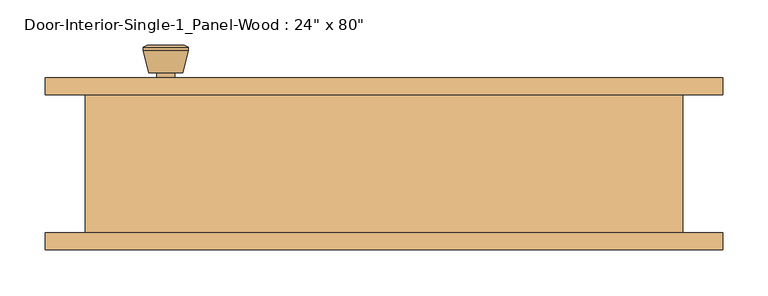
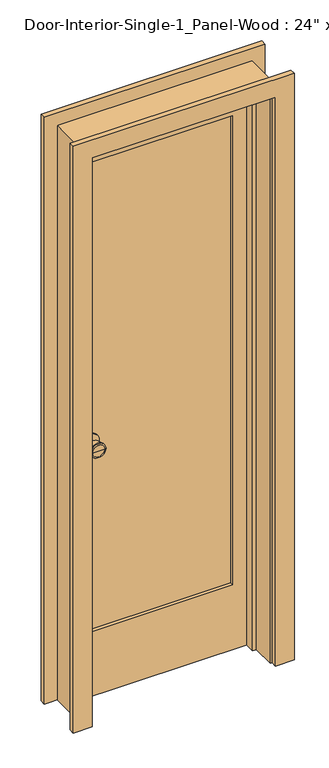
"""IFC4 building model written with IfcOpenShell, lengths in millimetres: door geometry."""

from ifc_helpers import new_model, si_unit, point, frame, frame_2d, origin, place, context, project, spatial, polyline, circle_curve, trimmed, segment, composite_curve, outline, extrude, faceted_brep, source, transform, mapped, element, save
from ifc_brep_helpers import plane_surface, cylinder_surface, revolved_surface, advanced_brep


def door_6ed77e8d(model_context):
    return source(origin(), model_context, "Body", "SolidModel", [
        advanced_brep(
        [(-241.3, 32.1, 914.4), (-231.3, 32.1, 914.4), (-251.3, 32.1, 914.4), (-220.8241324, -16.9, 914.4), (-241.3, -16.9, 914.4), (-261.7758676, -16.9, 914.4), (-216.3, -15.0721319, 914.4), (-266.3, -15.0721319, 914.4), (-216.3, -11.6084537, 914.4), (-266.3, -11.6084537, 914.4), (-222.663764, 13.1, 914.4), (-259.936236, 13.1, 914.4), (-231.3, 13.1, 914.4), (-251.3, 13.1, 914.4)],
        [
            (0, 1),
            (1, 2, circle_curve(frame((-241.3, 32.1, 914.4), z_axis=(0.0, 1.0, 0.0), x_axis=(-1.0, 0.0, 0.0)), 10.0)),
            (2, 0),
            (2, 1, circle_curve(frame((-241.3, 32.1, 914.4), z_axis=(0.0, 1.0, 0.0), x_axis=(-1.0, 0.0, 0.0)), 10.0)),
            (3, 4),
            (4, 5),
            (5, 3, circle_curve(frame((-241.3, -16.9, 914.4), z_axis=(0.0, -1.0, 0.0), x_axis=(-1.0, 0.0, 0.0)), 20.4758676)),
            (3, 5, circle_curve(frame((-241.3, -16.9, 914.4), z_axis=(0.0, -1.0, 0.0), x_axis=(-1.0, 0.0, 0.0)), 20.4758676)),
            (6, 3),
            (5, 7),
            (7, 6, circle_curve(frame((-241.3, -15.0721319, 914.4), z_axis=(0.0, -1.0, 0.0), x_axis=(-1.0, 0.0, 0.0)), 25.0)),
            (6, 7, circle_curve(frame((-241.3, -15.0721319, 914.4), z_axis=(0.0, -1.0, 0.0), x_axis=(-1.0, 0.0, 0.0)), 25.0)),
            (8, 6),
            (7, 9),
            (9, 8, circle_curve(frame((-241.3, -11.6084537, 914.4), z_axis=(0.0, -1.0, 0.0), x_axis=(-1.0, 0.0, 0.0)), 25.0)),
            (8, 9, circle_curve(frame((-241.3, -11.6084537, 914.4), z_axis=(0.0, -1.0, 0.0), x_axis=(-1.0, 0.0, 0.0)), 25.0)),
            (10, 8),
            (9, 11),
            (11, 10, circle_curve(frame((-241.3, 13.1, 914.4), z_axis=(0.0, -1.0, 0.0), x_axis=(-1.0, 0.0, 0.0)), 18.636236)),
            (10, 11, circle_curve(frame((-241.3, 13.1, 914.4), z_axis=(0.0, -1.0, 0.0), x_axis=(-1.0, 0.0, 0.0)), 18.636236)),
            (12, 10),
            (11, 13),
            (13, 12, circle_curve(frame((-241.3, 13.1, 914.4), z_axis=(0.0, -1.0, 0.0), x_axis=(-1.0, 0.0, 0.0)), 10.0)),
            (12, 13, circle_curve(frame((-241.3, 13.1, 914.4), z_axis=(0.0, -1.0, 0.0), x_axis=(-1.0, 0.0, 0.0)), 10.0)),
            (1, 12),
            (13, 2),
        ],
        [
            plane_surface(frame((-241.3, 32.1, 914.4), z_axis=(0.0, 1.0, 0.0), x_axis=(-1.0, 0.0, 0.0))),
            plane_surface(frame((-241.3, -16.9, 914.4), z_axis=(0.0, -1.0, 0.0), x_axis=(-1.0, 0.0, 0.0))),
            revolved_surface(polyline([(-261.7758676, -16.9, 914.4), (-266.3, -15.0721319, 914.4)]), (-241.3, 32.1, 914.4), (0.0, 1.0, 0.0)),
            cylinder_surface(frame((-241.3, 32.1, 914.4), z_axis=(0.0, 1.0, 0.0), x_axis=(-1.0, 0.0, 0.0)), 25.0),
            revolved_surface(polyline([(-266.3, -11.6084537, 914.4), (-259.936236, 13.1, 914.4)]), (-241.3, 32.1, 914.4), (0.0, 1.0, 0.0)),
            plane_surface(frame((-241.3, 13.1, 914.4), z_axis=(0.0, 1.0, 0.0), x_axis=(-1.0, 0.0, 0.0))),
            cylinder_surface(frame((-241.3, 32.1, 914.4), z_axis=(0.0, 1.0, 0.0), x_axis=(-1.0, 0.0, 0.0)), 10.0),
        ],
        [
            (0, [[1, 2, 3]]),
            (0, [[-3, 4, -1]]),
            (1, [[5, 6, 7]]),
            (1, [[-6, -5, 8]]),
            (2, [[9, -7, 10, 11]]),
            (2, [[-10, -8, -9, 12]]),
            (3, [[13, -11, 14, 15]]),
            (3, [[-14, -12, -13, 16]]),
            (4, [[17, -15, 18, 19]]),
            (4, [[-18, -16, -17, 20]]),
            (5, [[21, -19, 22, 23]]),
            (5, [[-22, -20, -21, 24]]),
            (6, [[25, -23, 26, -2]]),
            (6, [[-26, -24, -25, -4]]),
        ],
    ),
        extrude(outline(composite_curve([segment(trimmed(circle_curve(frame_2d((914.4, -241.3)), 30.0), [point((914.4, -271.3))], [point((914.4, -211.3))], False, "CARTESIAN"), True, "CONTINUOUS"), segment(trimmed(circle_curve(frame_2d((914.4, -241.3)), 30.0), [point((914.4, -211.3))], [point((914.4, -271.3))], False, "CARTESIAN"), True, "CONTINUOUS")], self_intersect=False)), frame((0.0, 32.1, 0.0), z_axis=(0.0, 1.0, 0.0), x_axis=(0.0, 0.0, 1.0)), (0.0, 0.0, 1.0), 6.0),
        advanced_brep(
        [(-241.3, 79.025, 914.4), (-251.3, 79.025, 914.4), (-231.3, 79.025, 914.4), (-220.8241324, 128.025, 914.4), (-261.7758676, 128.025, 914.4), (-241.3, 128.025, 914.4), (-216.3, 126.1971319, 914.4), (-266.3, 126.1971319, 914.4), (-216.3, 122.7334537, 914.4), (-266.3, 122.7334537, 914.4), (-222.663764, 98.025, 914.4), (-259.936236, 98.025, 914.4), (-231.3, 98.025, 914.4), (-251.3, 98.025, 914.4)],
        [
            (0, 1),
            (1, 2, circle_curve(frame((-241.3, 79.025, 914.4), z_axis=(0.0, -1.0, 0.0), x_axis=(-1.0, 0.0, 0.0)), 10.0)),
            (2, 0),
            (2, 1, circle_curve(frame((-241.3, 79.025, 914.4), z_axis=(0.0, -1.0, 0.0), x_axis=(-1.0, 0.0, 0.0)), 10.0)),
            (3, 4, circle_curve(frame((-241.3, 128.025, 914.4), z_axis=(0.0, 1.0, 0.0), x_axis=(-1.0, 0.0, 0.0)), 20.4758676)),
            (4, 5),
            (5, 3),
            (4, 3, circle_curve(frame((-241.3, 128.025, 914.4), z_axis=(0.0, 1.0, 0.0), x_axis=(-1.0, 0.0, 0.0)), 20.4758676)),
            (6, 7, circle_curve(frame((-241.3, 126.1971319, 914.4), z_axis=(0.0, 1.0, 0.0), x_axis=(-1.0, 0.0, 0.0)), 25.0)),
            (7, 4),
            (3, 6),
            (7, 6, circle_curve(frame((-241.3, 126.1971319, 914.4), z_axis=(0.0, 1.0, 0.0), x_axis=(-1.0, 0.0, 0.0)), 25.0)),
            (8, 9, circle_curve(frame((-241.3, 122.7334537, 914.4), z_axis=(0.0, 1.0, 0.0), x_axis=(-1.0, 0.0, 0.0)), 25.0)),
            (9, 7),
            (6, 8),
            (9, 8, circle_curve(frame((-241.3, 122.7334537, 914.4), z_axis=(0.0, 1.0, 0.0), x_axis=(-1.0, 0.0, 0.0)), 25.0)),
            (10, 11, circle_curve(frame((-241.3, 98.025, 914.4), z_axis=(0.0, 1.0, 0.0), x_axis=(-1.0, 0.0, 0.0)), 18.636236)),
            (11, 9),
            (8, 10),
            (11, 10, circle_curve(frame((-241.3, 98.025, 914.4), z_axis=(0.0, 1.0, 0.0), x_axis=(-1.0, 0.0, 0.0)), 18.636236)),
            (12, 13, circle_curve(frame((-241.3, 98.025, 914.4), z_axis=(0.0, 1.0, 0.0), x_axis=(-1.0, 0.0, 0.0)), 10.0)),
            (13, 11),
            (10, 12),
            (13, 12, circle_curve(frame((-241.3, 98.025, 914.4), z_axis=(0.0, 1.0, 0.0), x_axis=(-1.0, 0.0, 0.0)), 10.0)),
            (1, 13),
            (12, 2),
        ],
        [
            plane_surface(frame((-241.3, 79.025, 914.4), z_axis=(0.0, -1.0, 0.0), x_axis=(-1.0, 0.0, 0.0))),
            plane_surface(frame((-241.3, 128.025, 914.4), z_axis=(0.0, 1.0, 0.0), x_axis=(-1.0, 0.0, 0.0))),
            revolved_surface(polyline([(-261.7758676, 128.025, 914.4), (-266.3, 126.1971319, 914.4)]), (-241.3, 79.025, 914.4), (0.0, -1.0, 0.0)),
            cylinder_surface(frame((-241.3, 79.025, 914.4), z_axis=(0.0, -1.0, 0.0), x_axis=(-1.0, 0.0, 0.0)), 25.0),
            revolved_surface(polyline([(-266.3, 122.7334537, 914.4), (-259.936236, 98.025, 914.4)]), (-241.3, 79.025, 914.4), (0.0, -1.0, 0.0)),
            plane_surface(frame((-241.3, 98.025, 914.4), z_axis=(0.0, -1.0, 0.0), x_axis=(-1.0, 0.0, 0.0))),
            cylinder_surface(frame((-241.3, 79.025, 914.4), z_axis=(0.0, -1.0, 0.0), x_axis=(-1.0, 0.0, 0.0)), 10.0),
        ],
        [
            (0, [[1, 2, 3]]),
            (0, [[-3, 4, -1]]),
            (1, [[5, 6, 7]]),
            (1, [[8, -7, -6]]),
            (2, [[9, 10, -5, 11]]),
            (2, [[12, -11, -8, -10]]),
            (3, [[13, 14, -9, 15]]),
            (3, [[16, -15, -12, -14]]),
            (4, [[17, 18, -13, 19]]),
            (4, [[20, -19, -16, -18]]),
            (5, [[21, 22, -17, 23]]),
            (5, [[24, -23, -20, -22]]),
            (6, [[-2, 25, -21, 26]]),
            (6, [[-4, -26, -24, -25]]),
        ],
    ),
        extrude(outline(composite_curve([segment(trimmed(circle_curve(frame_2d((914.4, -241.3)), 30.0), [point((914.4, -271.3))], [point((914.4, -211.3))], False, "CARTESIAN"), True, "CONTINUOUS"), segment(trimmed(circle_curve(frame_2d((914.4, -241.3)), 30.0), [point((914.4, -211.3))], [point((914.4, -271.3))], False, "CARTESIAN"), True, "CONTINUOUS")], self_intersect=False)), frame((0.0, 73.025, 0.0), z_axis=(0.0, 1.0, 0.0), x_axis=(0.0, 0.0, 1.0)), (0.0, 0.0, 1.0), 6.0),
        extrude(outline(polyline([(244.475, 49.7416667), (-244.475, 49.7416667), (-244.475, 61.3833333), (244.475, 61.3833333), (244.475, 49.7416667)])), frame((0.0, 0.0, 231.775), z_axis=(0.0, 0.0, 1.0), x_axis=(1.0, 0.0, 0.0)), (0.0, 0.0, 1.0), 1681.1625),
        extrude(outline(polyline([(2032.0, -304.8), (0.0, -304.8), (0.0, 304.8), (2032.0, 304.8), (2032.0, -304.8)]), holes=[polyline([(1912.9375, -244.475), (1912.9375, 244.475), (231.775, 244.475), (231.775, -244.475), (1912.9375, -244.475)])]), frame((0.0, 38.1, 0.0), z_axis=(0.0, 1.0, 0.0), x_axis=(0.0, 0.0, 1.0)), (0.0, 0.0, 1.0), 34.925),
        faceted_brep([(330.2, 73.025, 0.0), (330.2, -79.375, 0.0), (304.8, -79.375, 0.0), (304.8, 3.175, 0.0), (292.1, 3.175, 0.0), (292.1, 38.1, 0.0), (304.8, 38.1, 0.0), (304.8, 73.025, 0.0), (330.2, 73.025, 2057.4), (330.2, -79.375, 2057.4), (-330.2, -79.375, 2057.4), (-330.2, -79.375, 0.0), (-304.8, -79.375, 0.0), (-304.8, -79.375, 2032.0), (304.8, -79.375, 2032.0), (304.8, 3.175, 2032.0), (-304.8, 3.175, 2032.0), (-304.8, 3.175, 0.0), (-292.1, 3.175, 0.0), (-292.1, 3.175, 2019.3), (292.1, 3.175, 2019.3), (292.1, 38.1, 2019.3), (-292.1, 38.1, 2019.3), (-292.1, 38.1, 0.0), (-304.8, 38.1, 0.0), (-304.8, 38.1, 2032.0), (304.8, 38.1, 2032.0), (304.8, 73.025, 2032.0), (-304.8, 73.025, 2032.0), (-304.8, 73.025, 0.0), (-330.2, 73.025, 0.0), (-330.2, 73.025, 2057.4)], [[[0, 1, 2, 3, 4, 5, 6, 7]], [[1, 0, 8, 9]], [[2, 1, 9, 10, 11, 12, 13, 14]], [[3, 2, 14, 15]], [[4, 3, 15, 16, 17, 18, 19, 20]], [[5, 4, 20, 21]], [[6, 5, 21, 22, 23, 24, 25, 26]], [[7, 6, 26, 27]], [[0, 7, 27, 28, 29, 30, 31, 8]], [[9, 8, 31, 10]], [[15, 14, 13, 16]], [[21, 20, 19, 22]], [[27, 26, 25, 28]], [[30, 29, 24, 23, 18, 17, 12, 11]], [[10, 31, 30, 11]], [[16, 13, 12, 17]], [[22, 19, 18, 23]], [[28, 25, 24, 29]]]),
        extrude(outline(polyline([(0.0, 311.15), (0.0, 374.65), (2101.85, 374.65), (2101.85, -374.65), (0.0, -374.65), (0.0, -311.15), (2038.35, -311.15), (2038.35, 311.15), (0.0, 311.15)])), frame((0.0, -98.425, 0.0), z_axis=(0.0, 1.0, 0.0), x_axis=(0.0, 0.0, 1.0)), (0.0, 0.0, 1.0), 19.05),
        extrude(outline(polyline([(0.0, 311.15), (0.0, 374.65), (2101.85, 374.65), (2101.85, -374.65), (0.0, -374.65), (0.0, -311.15), (2038.35, -311.15), (2038.35, 311.15), (0.0, 311.15)])), frame((0.0, 73.025, 0.0), z_axis=(0.0, 1.0, 0.0), x_axis=(0.0, 0.0, 1.0)), (0.0, 0.0, 1.0), 19.05),
    ])


if __name__ == "__main__":
    model = new_model("IFC4")
    model_context = context("Model", 3, world=origin())
    ifc_project = project(units=[si_unit("LENGTHUNIT", "METRE", prefix="MILLI")], contexts=[model_context])
    site = spatial("IfcSite", under=ifc_project)
    building = spatial("IfcBuilding", under=site)
    placement = place(None, origin())
    door_shape = door_6ed77e8d(model_context)
    element("IfcDoor", 1, ObjectType="Door-Interior-Single-1_Panel-Wood : 24\" x 80\"", at=placement, inside=building, context=model_context, shape_type="MappedRepresentation", body=[
        mapped(door_shape, transform((0.0, 0.0, 0.0), x_axis=(1.0, 0.0, 0.0), y_axis=(0.0, 1.0, 0.0), z_axis=(0.0, 0.0, 1.0))),
    ])
    save(model, "model.ifc")

# Revit data of these elements
# Type "Door-Interior-Single-1_Panel-Wood : 24\" x 80\""
#   Type Mark = "12"
#   Assembly Code = "C1020300"
#   Analytic Construction = "Wooden"
#   Top Rail = 0' - 4 11/16"
#   Thickness = 0' - 1 3/8"
#   Thermal Resistance (R) = 2.5876 (h·ft²·°F)/BTU
#   Swing Angle [instance default] = 90.00°
#   Stiles = 0' - 2 3/8"
#   Rough Width = 2' - 2"
#   Rough Height = 6' - 9"
#   Height = 6' - 8"
#   Width = 2' - 0"
#   Heat Transfer Coefficient (U) = 0.3865 BTU/(h·ft²·°F)
#   Bottom Rail = 0' - 9 1/8"
#   Trim Material = Cherry
#   Panel Material = Cherry
#   Frame Material = Cherry
#   Door Handle Material = Aluminum
#   Visual Light Transmittance = 0
#   Solar Heat Gain Coefficient = 0
#   Wall Closure = (empty or 0)
#   Function = (empty or 0)
# Element 1 (IfcDoor, "Door-Interior-Single-1_Panel-Wood : 24\" x 80\"")
#   Materials on its faces: "Cherry", "Aluminum"
# Materials
#   "Cherry": class "Wood", colour RGB 226 177 128, transparency 0, Description = "Prunus Serotina", Cost = 0
#   "Aluminum": class "Metal", colour RGB 247 247 247, transparency 0, Description = "Aluminum 6061", Cost = 0
